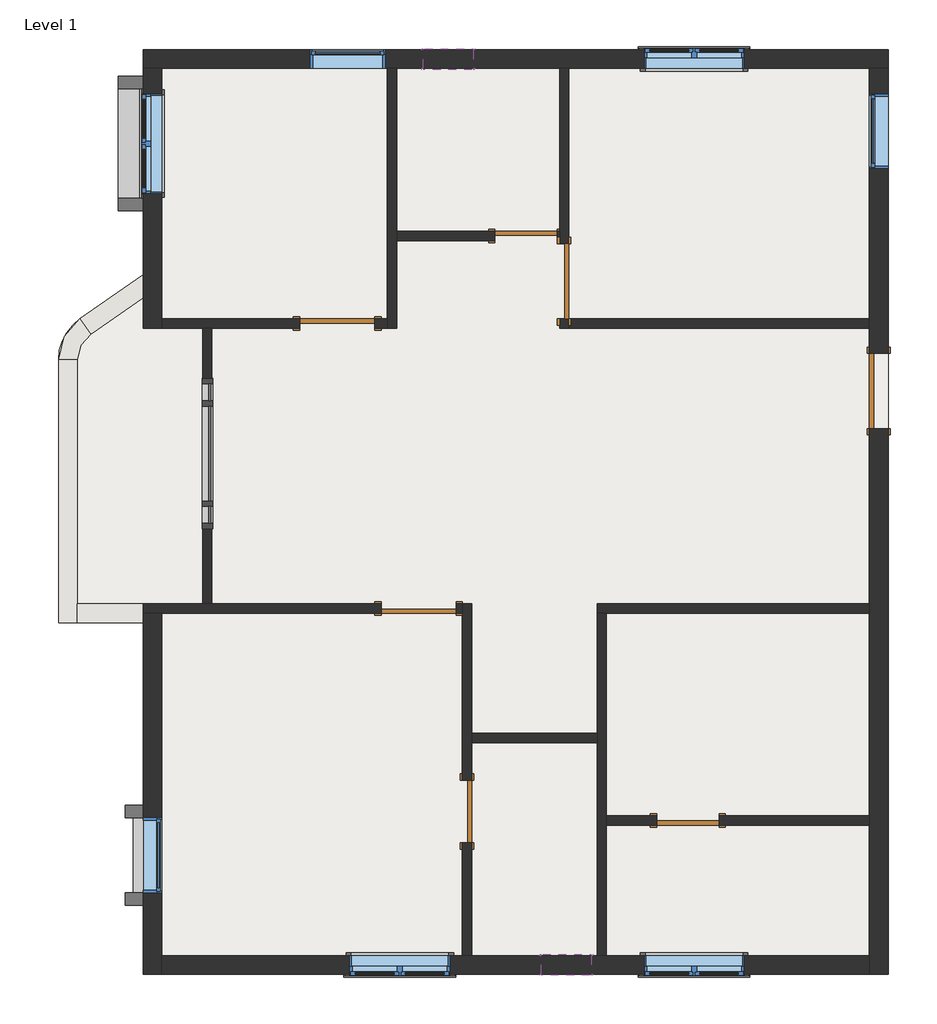
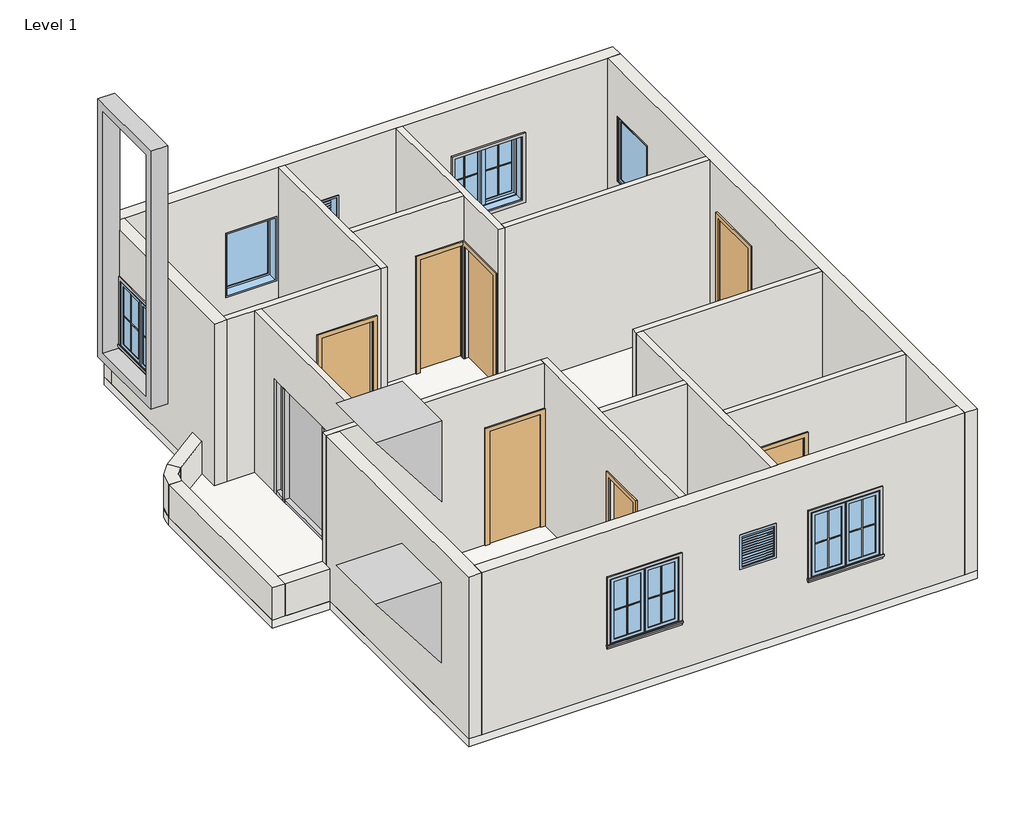
# One storey: 21 walls, 18 proxies, 9 windows, 7 doors, 7 members, 3 plates, 1 slab.
# Revit data of these elements (continued)
# Materials (continued)
#   "Default Floor": colour RGB 128 128 128, transparency 0, Cost = 0
#   "Default Wall": colour RGB 128 128 128, transparency 0, Cost = 0
# Room at (-8392.259, -2788.477) mm, phase "New Construction", upper level "Level 1", upper offset 10' - 0", lower offset 0' - 0"
#   Number = "KITCHEN"
#   Name = "Room"
# Room at (-14000.01, 3787.269) mm, phase "New Construction", upper level "Level 1", upper offset 10' - 0", lower offset 0' - 0"
#   Number = "STUDY"
#   Name = "Room"
# Room at (-11498.789, 4483.067) mm, phase "New Construction", upper level "Level 1", upper offset 10' - 0", lower offset 0' - 0"
#   Number = ""
#   Name = "TOILET"
# Room at (-8633.729, 3556.57) mm, phase "New Construction", upper level "Level 1", upper offset 10' - 0", lower offset 0' - 0"
#   Number = "BEDROOM-1"
#   Name = "Room"
# Room at (-15506.005, 384.633) mm, phase "New Construction", upper level "Level 1", upper offset 10' - 0", lower offset 0' - 0"
#   Name = "Room"
# Room at (-13677.205, -3707.253) mm, phase "New Construction", upper level "Level 1", upper offset 10' - 0", lower offset 0' - 0"
#   Number = "M-BEDROOM"
#   Name = "Room"
# Room at (-8046.257, -4610.869) mm, phase "New Construction", upper level "Level 1", upper offset 10' - 0", lower offset 0' - 0"
#   Number = "UTILITY"
#   Name = "Room"
# Room at (-10730.076, -4368.047) mm, phase "New Construction", upper level "Level 1", upper offset 10' - 0", lower offset 0' - 0"
#   Number = "M-TOILET"
#   Name = "Room"
# Room at (-10730.076, 384.633) mm, phase "New Construction", upper level "Level 1", upper offset 10' - 0", lower offset 0' - 0"
#   Name = "Room"
# Room at (-11021.003, -1895.634) mm, phase "New Construction", upper level "Level 1", upper offset 10' - 0", lower offset 0' - 0"
#   Number = "10"
